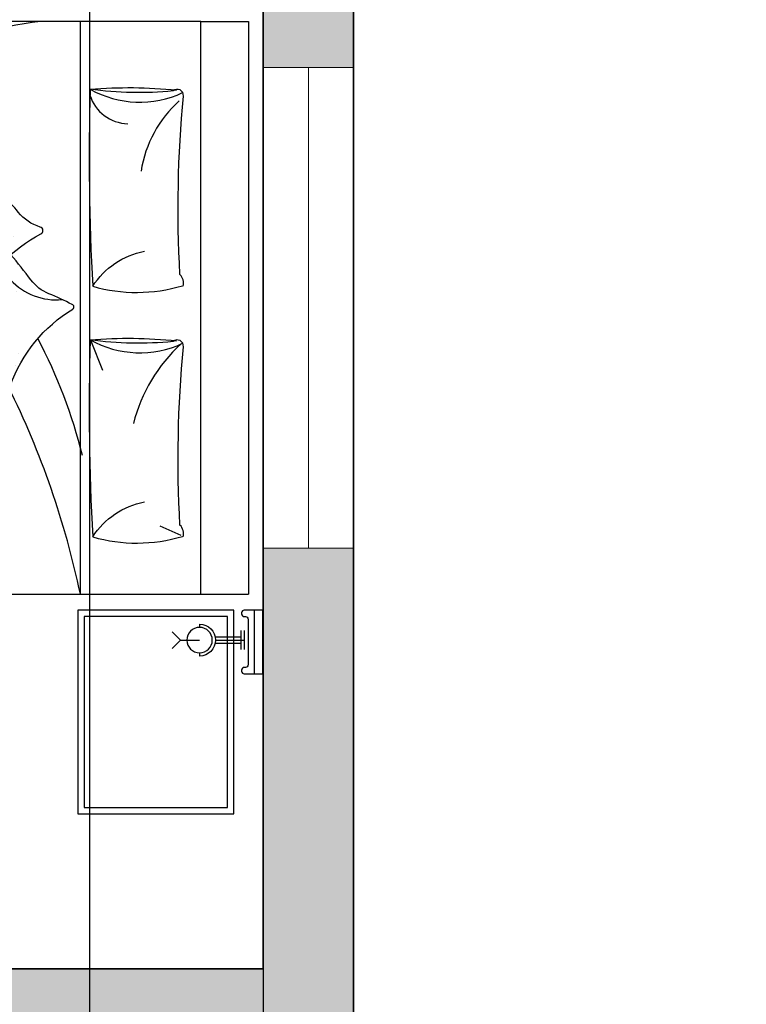
# Model space of a CAD drawing. Units: inches. Extents: x 3592 to 4861, y 1650 to 2243.
# Tile 16 of 30: x 4365 to 4438, y 1772 to 1870. Entities that reach past the tile are written whole.
import ezdxf

# ---------------------------------------------------------------- set-up
doc = ezdxf.new("R2010")
doc.units = ezdxf.units.IN
for name, color, linetype, lineweight in [('A-ANNO-DIMS', 2, 'Continuous', 13), ('A-FURN', 9, 'Continuous', 13), ('A-GLAZ', 4, 'Continuous', 18), ('A-WALL', 7, 'Continuous', 35)]:
    doc.layers.add(name, color=color, linetype=linetype, lineweight=lineweight)
doc.layers.add('A-WALL-PATT', color=252, linetype='Continuous', lineweight=13, true_color=0x939598)
for name, color, linetype in [('CEIL', 4, 'Continuous'), ('ELEC', 4, 'Continuous'), ('FUR', 42, 'Continuous'), ('wood', 26, 'Continuous')]:
    doc.layers.add(name, color=color, linetype=linetype)
doc.styles.get("Standard").update_dxf_attribs({"font": 'arial.ttf'})
doc.dimstyles.new('ISO-25', dxfattribs={"dimtxt": 9, "dimasz": 2.5, "dimexe": 1.25, "dimexo": 0.625, "dimtad": 1, "dimlunit": 3, "dimtxsty": 'Standard', "dimcen": 2.5, "dimadec": 0, "dimazin": 0, "dimtfac": 1, "dimtmove": 0, "dimatfit": 3, "dimfxl": 1, "dimarcsym": 0})

# ---------------------------------------------------------------- blocks, each defined once
blk = doc.blocks.new('*X20')
at = {"color": 0}
for p, q in [((3155.9, 8182.9), (3155.9, 8182.9)), ((3147.8, 8143.4), (3147.8, 8143.4)), ((3283, 8049.6), (3283, 8049.6)), ((3209.5, 8023.9), (3209.5, 8023.9)), ((3251.6, 7997), (3251.6, 7997)), ((3154.1, 7950.7), (3154.1, 7950.7))]:
    blk.add_line(p, q, dxfattribs=at)
blk = doc.blocks.new('*X19')
at = {"color": 0}
for p, q in [((3155.9, 8182.9), (3155.9, 8182.9)), ((3139.8, 7939.7), (3139.8, 7939.7))]:
    blk.add_line(p, q, dxfattribs=at)
blk = doc.blocks.new('*X18')
at = {"color": 0}
for p, q in [((3155.9, 8182.9), (3155.9, 8182.9)), ((3139.8, 7939.7), (3139.8, 7939.7))]:
    blk.add_line(p, q, dxfattribs=at)
blk = doc.blocks.new('*X17')
at = {"color": 0}
for p, q in [((3163, 7776.2), (3163, 7776.2)), ((3422.2, 7761.3), (3422.2, 7761.3)), ((3236.2, 7675.7), (3236.2, 7675.7)), ((3244.3, 7698.6), (3244.3, 7698.6)), ((3340.3, 7689.4), (3340.3, 7689.4))]:
    blk.add_line(p, q, dxfattribs=at)
blk = doc.blocks.new('BED1')
for p, q in [((0, -1000), (0, 800)), ((150, 800), (0, 800)), ((150, 800), (150, -1000)), ((2058.7, 800), (150, 800)), ((528, 800), (528, -1000)), ((211.8, 614.9), (277.5, 585.4)), ((2537.2, 404.9), (2237.2, 404.9)), ((2187.2, 354.9), (2187.2, -545.1)), ((2587.2, -545.1), (2587.2, 354.9)), ((2582, 188.1), (2565.4, 174.8)), ((2566.3, 178.5), (2565.2, 177.4)), ((2565.4, 174.8), (2585.7, 165.4)), ((2566.3, -296.8), (2565.2, -297.9)), ((2582, -287.1), (2565.4, -300.5)), ((2565.4, -300.5), (2585.7, -309.9)), ((2237.2, -595.1), (2537.2, -595.1)), ((150, -1000), (0, -1000)), ((150, -1000), (2063.5, -1000))]:
    blk.add_line(p, q)
for points in [[(934, 797.9), (930.9, 797.7), (928.3, 797.4), (926.3, 796.9), (924.9, 796.3), (923.8, 795.6), (923.1, 794.8), (922.7, 793.8), (922.5, 792.7), (922.4, 791.5), (922.5, 790.3), (922.6, 789.2), (922.6, 788.3), (922.6, 787.6), (922.4, 787.3), (922, 787.4), (921.4, 787.9), (920.6, 788.9), (919.5, 790.2), (918.4, 791.6), (917.1, 793.1), (915.9, 794.6), (914.6, 796), (913.3, 797.1), (912.2, 797.9), (911.1, 798.3), (910.1, 798.4), (909.2, 798), (908.3, 797.1), (907.5, 795.8), (906.8, 793.9), (906, 791.4), (905.4, 788.5), (904.8, 785.2), (904.2, 781.7), (903.7, 778.4), (903.2, 775.4), (902.8, 772.9), (902.5, 771.3), (902.3, 770.6), (902.1, 771.2), (902, 772.8), (901.8, 775.2), (901.7, 778.1), (901.5, 781.5), (901.2, 785), (900.8, 788.4), (900.2, 791.5), (899.5, 794.1), (898.6, 796.2), (897.6, 797.9), (896.5, 799.2), (895.3, 800), (894.1, 800.5), (893, 800.7), (891.9, 800.5), (890.9, 800.1), (890, 799), (889.1, 797.1), (888.3, 794), (887.6, 789.3), (886.9, 782.9), (886.2, 774.2), (885.5, 763.1), (884.8, 749.5), (884.2, 734.2), (883.6, 718.3), (883, 702.8), (882.5, 688.8), (882, 677.5), (881.7, 669.8), (881.5, 666.9), (881.3, 669.4), (881.3, 676.7), (881.3, 687.8), (881.2, 701.5), (881.1, 716.8), (880.8, 732.6), (880.2, 748), (879.4, 761.8), (878.3, 773.2), (876.9, 782.2), (875.1, 789.2), (872.9, 794.4), (870.3, 798), (869, 799)], [(2150, -913.5), (2150, 723.2)], [(2327.6, 182.3), (2530, 185.9), (2550.8, 181.9), (2561.7, 179), (2566, 176.7), (2566.9, 174.4), (2566.3, 171.9), (2562, 169.2), (2550.3, 166.5), (2527.7, 163.9), (2490.6, 161.8), (2345.5, 160.2), (2317.8, 158.5)], [(494.7, 3.1), (458.9, 95.3)], [(2149.7, -259.9), (2150, -268.4), (2150.1, -274.1), (2150.1, -278.1), (2150, -281.4), (2149.8, -284), (2149.5, -286.1), (2149.1, -287.8), (2148.7, -289), (2148.1, -289.9), (2147.4, -290.5), (2146.6, -290.8), (2145.6, -291), (2144.6, -291), (2143.6, -291), (2142.7, -290.9), (2141.9, -290.9), (2141.4, -290.9), (2141.1, -291), (2141.2, -291.4), (2141.7, -291.9), (2142.5, -292.6), (2143.5, -293.4), (2144.7, -294.4), (2146, -295.4), (2147.2, -296.5), (2148.4, -297.6), (2149.3, -298.6), (2150, -299.6), (2150.3, -300.5), (2150.4, -301.3), (2150, -302.1), (2149.3, -302.8), (2148.2, -303.5), (2146.6, -304.1), (2144.6, -304.7), (2142.1, -305.2), (2139.3, -305.7), (2136.5, -306.2), (2133.7, -306.6), (2131.2, -307), (2129.2, -307.3), (2127.8, -307.6), (2127.3, -307.8), (2127.7, -308), (2129, -308.1), (2131, -308.2), (2133.5, -308.3), (2136.3, -308.5), (2139.2, -308.7), (2142, -309), (2144.6, -309.5), (2146.8, -310.1), (2148.6, -310.9), (2150, -311.7), (2151, -312.7), (2151.7, -313.6), (2152.1, -314.6), (2152.3, -315.6), (2152.2, -316.5), (2151.8, -317.3), (2150.9, -318.1), (2149.3, -318.8), (2146.7, -319.4), (2142.8, -320), (2137.4, -320.6), (2130.2, -321.2), (2121, -321.8), (2109.7, -322.3), (2096.9, -322.9), (2083.6, -323.4), (2070.7, -323.9), (2059.1, -324.3), (2049.6, -324.7), (2043.2, -325), (2040.8, -325.2), (2042.9, -325.3), (2049, -325.3), (2058.2, -325.3), (2069.6, -325.4), (2082.3, -325.5), (2095.6, -325.8), (2108.4, -326.2), (2119.9, -326.8), (2129.4, -327.8), (2136.9, -329), (2142.7, -330.5), (2147, -332.3), (2150, -334.4), (2150.9, -335.6)], [(2246.5, -294.4), (2530, -289.4), (2550.8, -293.4), (2561.7, -296.3), (2566, -298.6), (2566.9, -300.8), (2566.3, -303.4), (2562, -306.1), (2550.3, -308.8), (2527.7, -311.3), (2490.6, -313.5), (2345.5, -315), (2238.6, -321.8)], [(1733.7, -998.3), (1731.1, -998.1), (1729, -997.8), (1727.4, -997.4), (1726.1, -997), (1725.2, -996.4), (1724.7, -995.7), (1724.3, -994.8), (1724.1, -993.9), (1724.1, -992.9), (1724.1, -991.9), (1724.2, -991), (1724.2, -990.2), (1724.2, -989.7), (1724.1, -989.4), (1723.8, -989.5), (1723.2, -990), (1722.5, -990.8), (1721.7, -991.8), (1720.7, -993), (1719.7, -994.3), (1718.6, -995.5), (1717.5, -996.6), (1716.5, -997.6), (1715.5, -998.3), (1714.6, -998.6), (1713.8, -998.6), (1713, -998.3), (1712.3, -997.6), (1711.7, -996.5), (1711, -994.9), (1710.4, -992.9), (1709.9, -990.4), (1709.4, -987.6), (1708.9, -984.8), (1708.5, -982), (1708.1, -979.5), (1707.8, -977.4), (1707.5, -976.1), (1707.3, -975.5), (1707.1, -976), (1707, -977.3), (1706.9, -979.3), (1706.8, -981.8), (1706.7, -984.6), (1706.4, -987.5), (1706.1, -990.3), (1705.6, -992.9), (1705, -995.1), (1704.2, -996.9), (1703.4, -998.3), (1702.4, -999.3), (1701.5, -1000), (1700.5, -1000.4), (1699.6, -1000.6), (1698.7, -1000.4), (1697.8, -1000.1), (1697, -999.2), (1696.3, -997.6), (1695.7, -995), (1695.1, -991.1), (1694.5, -985.7), (1693.9, -978.5), (1693.3, -969.3), (1692.8, -957.9), (1692.2, -945.2), (1691.7, -931.9), (1691.2, -919), (1690.8, -907.4), (1690.4, -897.9), (1690.1, -891.5), (1689.9, -889.1), (1689.8, -891.2), (1689.8, -897.3), (1689.8, -906.5), (1689.7, -917.9), (1689.6, -930.6), (1689.4, -943.8), (1688.9, -956.6), (1688.3, -968.1), (1687.3, -977.6), (1686.1, -985.2), (1684.6, -991), (1682.8, -995.3), (1680.7, -998.3), (1679.6, -999.2)]]:
    blk.add_lwpolyline(points)
for points in [[(205.5, 619.6, 0.267769), (215.1, 582.4, -0.037739), (204.3, 21.8, 0.684696), (236.7, 5.5, -0.060702), (497.2, 0.1, -0.046649), (225.9, 3.1, -1.318436)], [(489.2, 619.6, 0.144019), (207.6, 617.9, 0.248643)], [(497.2, 0.1, 0.021276), (489.2, 619.6, -0.206383), (326.6, 509.4, 0.237198)], [(211.8, 12.8, 0.143972), (361.6, 262.9, 1.292232)], [(886.4, -150, -0.069098), (985, -66.5, 0.658965), (982.1, -48.7, -0.049789), (927.4, -29, -0.103757), (896.6, -5.4, 0.055725), (800.9, 83.3, -0.11866), (782.7, 104.9, 0.016811), (761.6, 143.9, 0.70791), (748.3, 144, -0.16964), (551.9, -96.6, 0.664036), (554, -110.7, 0.023706), (627, -144.7, -0.134834), (683.2, -188, 0.012748), (746.3, -267.4)], [(969.1, -259.1, 0.263265), (936.3, -236.9, -0.026108), (909.2, -233.2, 0.027613), (945.1, -234.2, -0.089259), (872.7, -120, 0.662242), (857.6, -119.3, -0.162037), (651.8, -332.7, 0.676499), (654, -354.5, -0.160513), (722.9, -401.5, 0.07473), (773.5, -450.3, -0.187721), (845.5, -559.9, 0.70791), (858.8, -561.4, -0.010003), (898.6, -497.3, -0.113819), (947.3, -450.2, 0.099539), (1032.5, -372.4, -0.173425), (1070.9, -346.4, 0.589988), (1076.2, -326.1, 0.137312), (923.9, -245.9, 0.137312)], [(489.2, -168.2, 0.144019), (207.6, -169.9, 0.248643)], [(205.5, -168.2, 0.267769), (215.1, -205.4, -0.037739), (204.3, -766, 0.684696), (236.7, -782.3, -0.060702), (497.2, -787.7, -0.046649), (225.9, -784.7, -1.318436)], [(497.2, -787.7, 0.021276), (489.2, -168.2, -0.206383), (326.6, -278.4, 0.237198)], [(1446, -733.4, -0.095039), (652.8, -1001.7)]]:
    blk.add_lwpolyline(points, format="xyb")
for centre, radius, start, end in [((3208.8, 1363.3), 2739.4, 191.8679, 206.3247), ((1608.1, 842.5), 496.3, 305.1901, 354.0206), ((2062.7, 713.7), 86.5, 0, 93.5376), ((1138.6, 793.9), 983.2, 294.6078, 358.3033), ((2237.2, 354.9), 50, 90, 180), ((2227.5, 373.5), 32.8, 17.833, 72.8005), ((2546.9, 373.5), 32.8, 107.1995, 162.167), ((2537.2, 354.9), 50, 0, 90), ((2321.1, 409.7), 84.5, 185.6196, 217.1396), ((2453.3, 409.7), 84.5, 322.8604, 354.3804), ((2098.7, 754.7), 1625, 193.905, 207.8169), ((2201.9, 323.3), 34.8, 50.8413, 114.9586), ((2212.2, 381.5), 36.5, 226.8095, 258.3841), ((2572.5, 323.3), 34.8, 65.0414, 129.1587), ((2562.2, 381.5), 36.5, 281.6159, 313.1905), ((751.8, 88.7), 34.9, 336.8352, 27.7218), ((684.2, 86), 100.3, 353.675, 10.882), ((1074.1, 198.8), 306.1, 197.8602, 241.5122), ((341.4, -277.7), 318.5, 60.7125, 115.009), ((983.7, -79.5), 20.8, 73.7967, 130.4566), ((978.5, -68.6), 14.3, 39.7097, 85.9506), ((602.5, -324), 198.6, 43.2035, 95.0556), ((3208.8, 1363.3), 2739.4, 212.9314, 216.951), ((981.1, -281.8), 131.1, 164.0372, 243.4536), ((980, -379), 163.4, 152.6104, 209.361), ((3208.8, 1363.3), 2739.4, 218.6329, 229.9449), ((2098.7, 754.7), 1625, 226.5887, 246.3156), ((3402.5, -342.9), 1408.5, 182.9917, 205.6819), ((2178, -513.5), 33, 286.1827, 338.1386), ((2188.1, -476.2), 73, 269.4513, 322.8027), ((-34.4, -471.2), 376.5, 312.0118, 350.9635), ((2237.2, -545.1), 50, 180, 270), ((2453.3, -600), 84.5, 5.6196, 37.1396), ((2537.2, -545.1), 50, 270, 0), ((2572.5, -513.6), 34.8, 230.8413, 294.9586), ((2562.2, -571.8), 36.5, 46.8095, 78.3841), ((2271.1, -580.9), 35.8, 148.9055, 197.5541), ((2546.9, -563.8), 32.8, 197.833, 252.8005), ((375.7, -807.4), 128.2, 17.4073, 88.5129), ((341.4, -1065.5), 318.5, 60.7125, 115.009), ((1929.1, -1126), 250.5, 37.8553, 88.4405), ((2063.5, -913.5), 86.5, 270, 0)]:
    blk.add_arc(centre, radius, start, end)
for name in ['*X19', '*X18', '*X20', '*X17']:
    blk.add_blockref(name, (-2425.3, -8101.4))
blk = doc.blocks.new('APLIQ')
at = {"layer": 'ELEC'}
for p, q in [((0, 0.2), (-0.0261, 0.2261)), ((0, 0.2), (0.0261, 0.2261)), ((0, 0.2), (0, 0.14)), ((-0.05, 0.14), (-0.04, 0.14)), ((0.04, 0.14), (0.05, 0.14)), ((-0.01, 0.09), (-0.01, 0.01)), ((0, 0.09), (0, 0)), ((0.01, 0.09), (0.01, 0.01)), ((-0.03, 0.01), (0.03, 0.01)), ((-0.03, 0), (0.03, 0))]:
    blk.add_line(p, q, dxfattribs=at)
blk.add_circle((0, 0.14), 0.04, dxfattribs=at)
blk.add_arc((0, 0.14), 0.05, 180, 0, dxfattribs=at)
blk = doc.blocks.new('A$C68AE1801')
at = {"layer": 'FUR'}
for points in [[(2.5416, 0), (2.5416, 0.64), (2.0516, 0.64), (2.0516, 0)], [(2.5216, 0.02), (2.5216, 0.62), (2.0716, 0.62), (2.0716, 0.02)]]:
    blk.add_lwpolyline(points, close=True, dxfattribs=at)
at = {"layer": 'wood'}
blk.add_line((2.6057, 0.44), (2.6057, 0.64), dxfattribs=at)
blk.add_lwpolyline([(2.5657, 0.452), (2.5657, 0.448, 0.414214), (2.5737, 0.44), (2.6321, 0.44), (2.6321, 0.64), (2.5737, 0.64, 0.414214), (2.5657, 0.632), (2.5657, 0.628, 0.414214), (2.5737, 0.62), (2.5777, 0.62, -0.414214), (2.5857, 0.612), (2.5857, 0.468, -0.414214), (2.5777, 0.46), (2.5737, 0.46, 0.414214)], format="xyb", close=True, dxfattribs=at)
at = {"layer": 'CEIL', "xscale": -1, "rotation": 90}
blk.add_blockref('APLIQ', (2.5736, 0.546), dxfattribs=at)
at = {"layer": 'FUR', "xscale": 0.001, "yscale": 0.001, "zscale": 0.001, "rotation": 180}
blk.add_blockref('BED1', (2.5872, 1.49), dxfattribs=at)
blk = doc.blocks.new('*D173')
at = {"layer": 'A-ANNO-DIMS', "color": 0, "lineweight": -2, "transparency": 16777216}
for p, q in [((4372.046, 2138.774), (4372.046, 1656.919)), ((4389.37, 2131.594), (4389.37, 1656.919)), ((4374.546, 1658.169), (4386.87, 1658.169)), ((4389.37, 1658.169), (4437.168, 1658.169))]:
    blk.add_line(p, q, dxfattribs=at)
at = {"layer": 'A-ANNO-DIMS', "color": 0, "transparency": 16777216}
for points in [[(4374.546, 1658.586), (4374.546, 1657.752), (4372.046, 1658.169)], [(4386.87, 1658.586), (4386.87, 1657.752), (4389.37, 1658.169)]]:
    blk.add_solid(points, dxfattribs=at)
at = {"layer": 'Defpoints', "color": 0, "transparency": 16777216}
for p in [(4372.046, 2139.399), (4389.37, 2132.219), (4389.37, 1658.169)]:
    blk.add_point(p, dxfattribs=at)
at = {"layer": 'A-ANNO-DIMS', "color": 0, "transparency": 16777216, "insert": (4414.519, 1663.447), "char_height": 9, "attachment_point": 5}
blk.add_mtext('1\'-5 1/2"', dxfattribs=at)

msp = doc.modelspace()

# ---------------------------------------------------------------- hatches: boundary and pattern name
at = {"layer": 'A-WALL-PATT'}
h = msp.add_hatch(color=256, dxfattribs=at)
h.dxf.hatch_style = 1
h.paths.add_polyline_path([(4398.37, 2165.219), (4038.37, 2165.219), (4038.37, 1993.219), (4047.37, 1993.219), (4047.37, 2156.219), (4191.37, 2156.219), (4191.37, 2150.219), (4195.37, 2150.219), (4195.37, 2156.219), (4256.37, 2156.219), (4256.37, 2150.219), (4265.37, 2150.219), (4265.37, 2156.219), (4389.37, 2156.219), (4389.37, 2114.219), (4398.37, 2114.219)])
h.paths.add_polyline_path([(4265.37, 2102.219), (4256.37, 2102.219), (4256.37, 2096.219), (4195.37, 2096.219), (4195.37, 2102.219), (4191.37, 2102.219), (4191.37, 2020.219), (4195.37, 2020.219), (4195.37, 2087.219), (4256.37, 2087.219), (4256.37, 2020.219), (4306.37, 2020.219), (4306.37, 2024.219), (4265.37, 2024.219)], flags=17)
h.paths.add_polyline_path([(4398.37, 2066.219), (4389.37, 2066.219), (4389.37, 2024.219), (4348.37, 2024.219), (4348.37, 2020.219), (4389.37, 2020.219), (4389.37, 1989.719), (4398.37, 1989.719)])
h.paths.add_polyline_path([(4398.37, 1941.719), (4389.37, 1941.719), (4389.37, 1911.219), (4301.37, 1911.219), (4301.37, 1907.219), (4389.37, 1907.219), (4389.37, 1865.219), (4398.37, 1865.219)])
h.paths.add_polyline_path([(4398.37, 1817.219), (4389.37, 1817.219), (4389.37, 1775.219), (4265.37, 1775.219), (4265.37, 1911.219), (4256.37, 1911.219), (4256.37, 1817.219), (4220.87, 1817.219), (4220.87, 1808.219), (4256.37, 1808.219), (4256.37, 1766.219), (4389.37, 1766.219), (4389.37, 1694.219), (4256.37, 1694.219), (4256.37, 1685.219), (4398.37, 1685.219)])
h.paths.add_polyline_path([(4178.87, 1817.219), (4077.37, 1817.219), (4077.37, 1808.219), (4178.87, 1808.219)])
h.paths.add_polyline_path([(4111.37, 2020.219), (4155.37, 2020.219), (4155.37, 2024.219), (4077.37, 2024.219), (4077.37, 2020.219), (4107.37, 2020.219), (4107.37, 1942.219), (4047.37, 1942.219), (4047.37, 1969.219), (4038.37, 1969.219), (4038.37, 1911.219), (4047.37, 1911.219), (4047.37, 1938.219), (4107.37, 1938.219), (4107.37, 1860.219), (4077.37, 1860.219), (4077.37, 1856.219), (4111.37, 1856.219)])
h.paths.add_polyline_path([(4047.37, 1887.219), (4038.37, 1887.219), (4038.37, 1685.219), (4152.37, 1685.219), (4152.37, 1715.219), (4143.37, 1715.219), (4143.37, 1694.219), (4047.37, 1694.219)])
h.paths.add_polyline_path([(4152.37, 1772.219), (4143.37, 1772.219), (4143.37, 1751.219), (4152.37, 1751.219)], flags=17)

# ---------------------------------------------------------------- linework, layer by layer
at = {"layer": 'A-GLAZ'}
for p, q in [((4389.37, 1865.219), (4398.37, 1865.219)), ((4393.87, 1865.219), (4393.87, 1817.219)), ((4389.37, 1817.219), (4398.37, 1817.219))]:
    msp.add_line(p, q, dxfattribs=at)
at = {"layer": 'A-WALL'}
for p, q in [((4398.37, 2165.219), (4398.37, 1685.219)), ((4389.37, 1907.219), (4389.37, 1775.219)), ((4389.37, 1775.219), (4265.37, 1775.219))]:
    msp.add_line(p, q, dxfattribs=at)

# ---------------------------------------------------------------- block references
at = {"layer": 'A-FURN', "xscale": 31.7658940618111, "yscale": 31.7658940618111, "zscale": 31.7658940618111}
msp.add_blockref('A$C68AE1801', (4305.708, 1790.711), dxfattribs=at)

# ---------------------------------------------------------------- dimensions: what is measured, and where the dimension line sits
at = {"layer": 'A-ANNO-DIMS'}
dim = msp.add_linear_dim(base=(4389.37, 1658.169), p1=(4372.046, 2139.399), p2=(4389.37, 2132.219), dimstyle='ISO-25', override={"dimdec": 1, "dimlfac": 1, "dimrnd": 0, "dimzin": 1, "dimdsep": 46, "dimlunit": 4, "dimfrac": 2}, dxfattribs=at)
dim.commit()
dim.dimension.update_dxf_attribs({"geometry": '*D173', "text_midpoint": (4414.519, 1663.447)})

doc.saveas('drawing.dxf')
